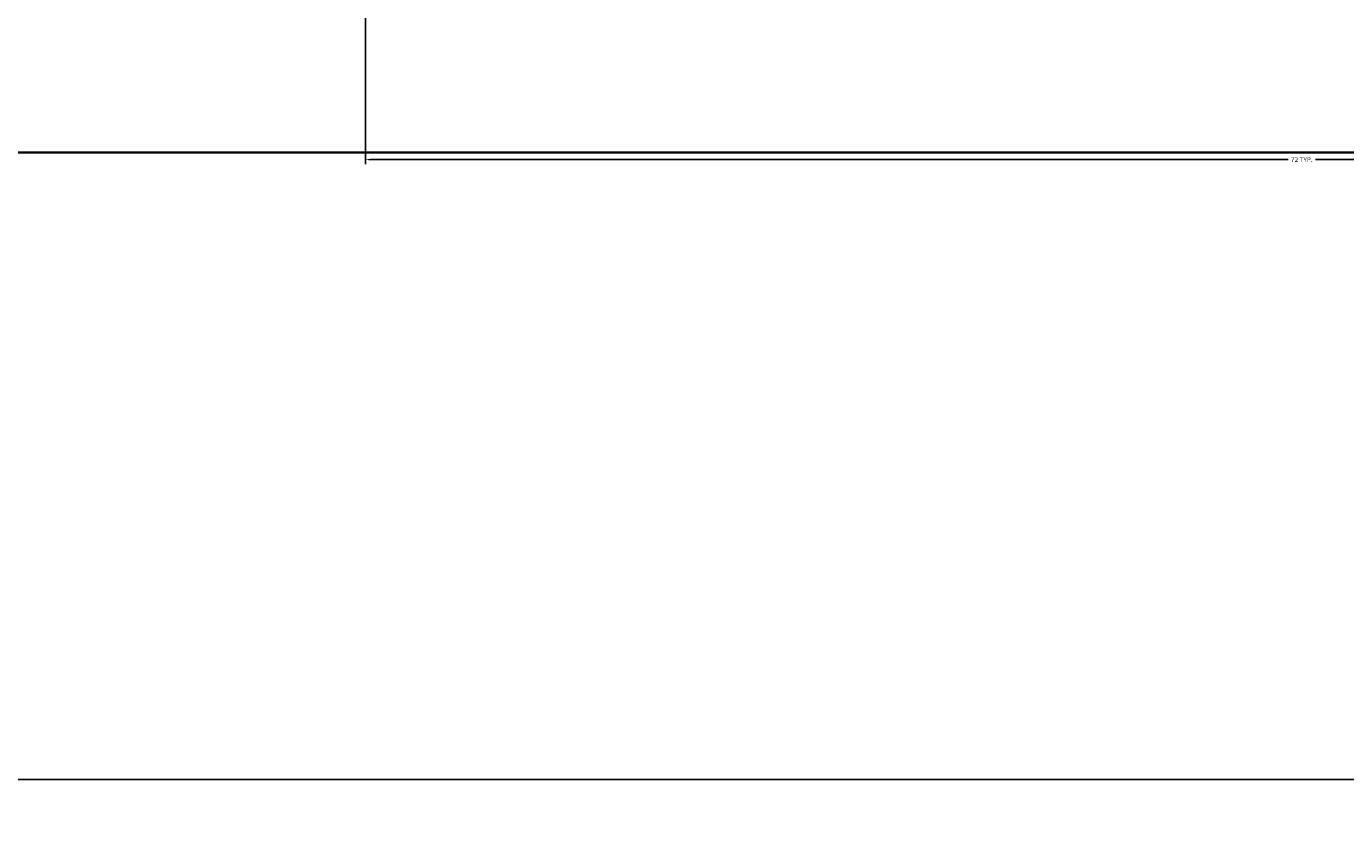
# Model space of a CAD drawing. Units: inches. Extents: x -61 to 1599, y -1316 to 257.
# Tile 3 of 204: x 99 to 149, y -1242 to -1211. Entities that reach past the tile are written whole.
import ezdxf

# ---------------------------------------------------------------- set-up
doc = ezdxf.new("R2010")
doc.units = ezdxf.units.IN
doc.header["$MEASUREMENT"] = 0
doc.layers.add('A-ANNO-DIMS', color=2, linetype='Continuous', lineweight=18)
doc.layers.add('WALLS', color=4, linetype='Continuous', lineweight=35)
doc.styles.get("Standard").update_dxf_attribs({"font": 'arial.ttf'})
doc.dimstyles.get("Standard").update_dxf_attribs({"dimtxt": 0.18, "dimasz": 0.18, "dimexe": 0.18, "dimexo": 0.0625, "dimgap": 0.09, "dimtad": 0, "dimtih": 1, "dimtoh": 1, "dimdec": 0, "dimzin": 0, "dimdsep": 46, "dimlunit": 3, "dimtxsty": 'Standard', "dimcen": 0.09, "dimadec": 0, "dimazin": 0, "dimtfac": 1, "dimtdec": 0, "dimtofl": 0, "dimtmove": 0, "dimatfit": 3, "dimfxl": 1, "dimtolj": 1, "dimtzin": 0, "dimarcsym": 0})

# ---------------------------------------------------------------- blocks, each defined once
blk = doc.blocks.new('*D635')
at = {"layer": 'A-ANNO-DIMS', "color": 0, "lineweight": -2, "transparency": 16777216}
for p, q in [((111.872, -1202.381), (111.872, -1216.391)), ((183.57, -1202.381), (183.57, -1216.391)), ((112.052, -1216.211), (147.193, -1216.211)), ((183.39, -1216.211), (148.248, -1216.211))]:
    blk.add_line(p, q, dxfattribs=at)
at = {"layer": 'A-ANNO-DIMS', "color": 0, "transparency": 16777216}
for points in [[(112.052, -1216.181), (112.052, -1216.241), (111.872, -1216.211)], [(183.39, -1216.181), (183.39, -1216.241), (183.57, -1216.211)]]:
    blk.add_solid(points, dxfattribs=at)
at = {"layer": 'DEFPOINTS', "color": 0, "transparency": 16777216}
for p in [(111.872, -1202.318), (183.57, -1202.318), (183.57, -1216.211)]:
    blk.add_point(p, dxfattribs=at)
at = {"layer": 'A-ANNO-DIMS', "color": 0, "transparency": 16777216, "insert": (147.721, -1216.211), "char_height": 0.18, "attachment_point": 5}
blk.add_mtext('\\A1;72 TYP.', dxfattribs=at)
blk = doc.blocks.new('*D687')
at = {"layer": 'A-ANNO-DIMS', "color": 0, "lineweight": -2, "transparency": 16777216}
for p, q in [((289.418, 181.677), (-61.077, 181.677)), ((-60.897, 181.497), (-60.897, -528.952)), ((-60.897, -1239.765), (-60.897, -529.316)), ((319.64, -1239.945), (-61.077, -1239.945))]:
    blk.add_line(p, q, dxfattribs=at)
at = {"layer": 'A-ANNO-DIMS', "color": 0, "transparency": 16777216}
for points in [[(-60.927, 181.497), (-60.867, 181.497), (-60.897, 181.677)], [(-60.927, -1239.765), (-60.867, -1239.765), (-60.897, -1239.945)]]:
    blk.add_solid(points, dxfattribs=at)
at = {"layer": 'DEFPOINTS', "color": 0, "transparency": 16777216}
for p in [(289.481, 181.677), (-60.897, -1239.945), (319.703, -1239.945)]:
    blk.add_point(p, dxfattribs=at)
at = {"layer": 'A-ANNO-DIMS', "color": 0, "transparency": 16777216, "insert": (-60.897, -529.134), "char_height": 0.18, "attachment_point": 5}
blk.add_mtext('\\A1;1421.6', dxfattribs=at)
blk = doc.blocks.new('*D688')
at = {"layer": 'A-ANNO-DIMS', "color": 0, "lineweight": -2, "transparency": 16777216}
for p, q in [((14.703, -1216.007), (14.703, -1315.725)), ((544.703, -1216.007), (544.703, -1315.725)), ((14.883, -1315.545), (279.414, -1315.545)), ((544.523, -1315.545), (279.991, -1315.545))]:
    blk.add_line(p, q, dxfattribs=at)
at = {"layer": 'A-ANNO-DIMS', "color": 0, "transparency": 16777216}
for points in [[(14.883, -1315.515), (14.883, -1315.575), (14.703, -1315.545)], [(544.523, -1315.515), (544.523, -1315.575), (544.703, -1315.545)]]:
    blk.add_solid(points, dxfattribs=at)
at = {"layer": 'DEFPOINTS', "color": 0, "transparency": 16777216}
for p in [(14.703, -1215.945), (544.703, -1215.945), (544.703, -1315.545)]:
    blk.add_point(p, dxfattribs=at)
at = {"layer": 'A-ANNO-DIMS', "color": 0, "transparency": 16777216, "insert": (279.703, -1315.545), "char_height": 0.18, "attachment_point": 5}
blk.add_mtext('\\A1;530', dxfattribs=at)

msp = doc.modelspace()

# ---------------------------------------------------------------- linework, layer by layer
at = {"layer": 'WALLS'}
msp.add_line((14.7028, -1215.9446), (237.7028, -1215.9446), dxfattribs=at)

# ---------------------------------------------------------------- dimensions: what is measured, and where the dimension line sits
at = {"layer": 'A-ANNO-DIMS'}
dim = msp.add_linear_dim(base=(-60.8972, -1239.9446), p1=(289.4807, 181.6771), p2=(319.7028, -1239.9446), angle=90, dimstyle='Standard', override={"dimdec": 1, "dimlfac": 1, "dimrnd": 0, "dimzin": 0, "dimdsep": 46, "dimlunit": 2}, dxfattribs=at)
dim.commit()
dim.dimension.update_dxf_attribs({"geometry": '*D687', "text_midpoint": (-60.8972, -529.1337)})
dim = msp.add_linear_dim(base=(183.5695, -1216.2111), p1=(111.8719, -1202.3182), p2=(183.5695, -1202.3182), text='<> TYP.', dimstyle='Standard', override={"dimdec": 0, "dimlfac": 1, "dimrnd": 0, "dimzin": 0, "dimdsep": 46, "dimlunit": 2}, dxfattribs=at)
dim.commit()
dim.dimension.update_dxf_attribs({"geometry": '*D635', "text_midpoint": (147.7207, -1216.2111)})
dim = msp.add_linear_dim(base=(544.7028, -1315.5446), p1=(14.7028, -1215.9446), p2=(544.7028, -1215.9446), dimstyle='Standard', override={"dimdec": 0, "dimlfac": 1, "dimrnd": 0, "dimzin": 0, "dimdsep": 46, "dimlunit": 2}, dxfattribs=at)
dim.commit()
dim.dimension.update_dxf_attribs({"geometry": '*D688', "text_midpoint": (279.7028, -1315.5446)})

doc.saveas('drawing.dxf')
